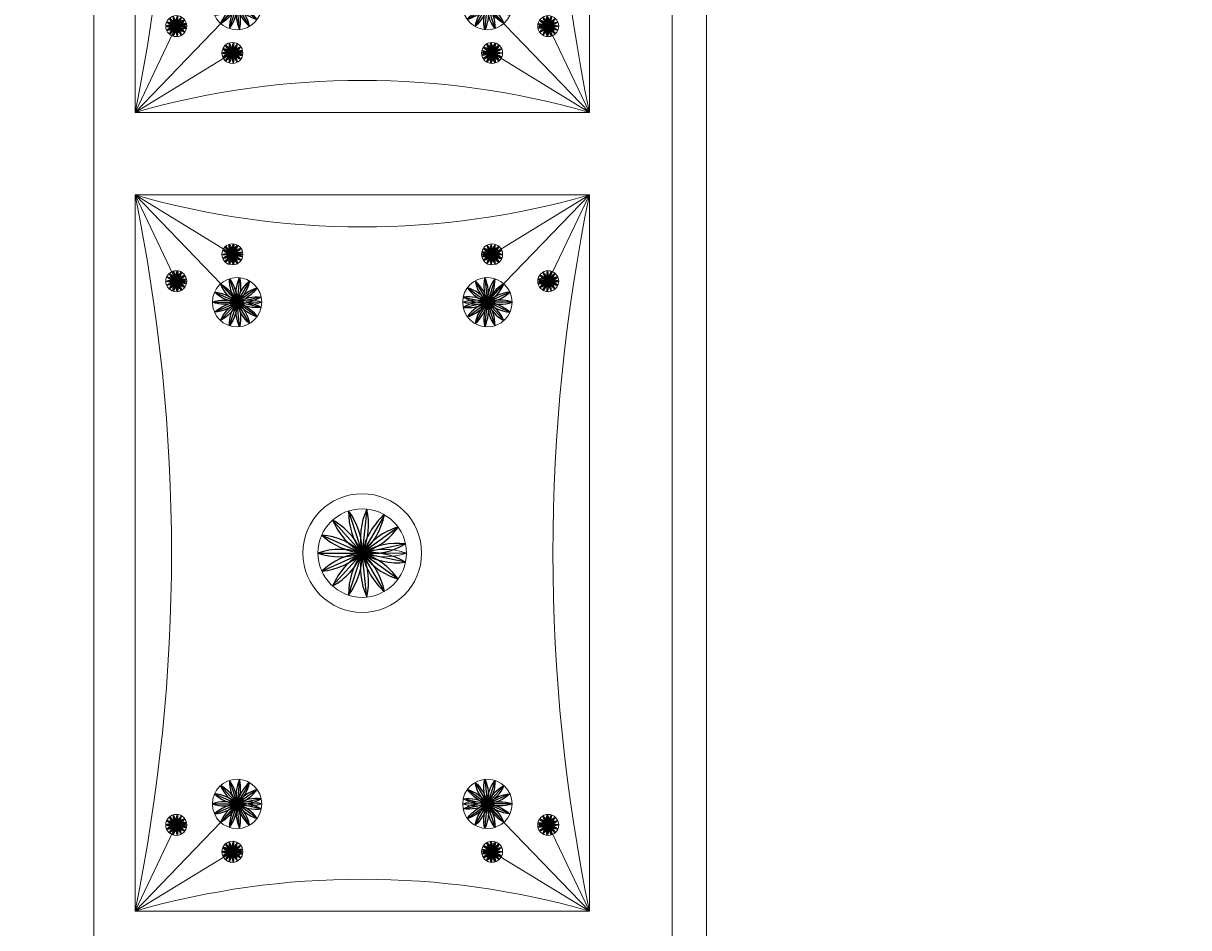
# Model space of a CAD drawing. Units: inches. Extents: x -61 to 1599, y -1316 to 257.
# Tile 147 of 204: x 406 to 440, y 74 to 101. Entities that reach past the tile are written whole.
import ezdxf

# ---------------------------------------------------------------- set-up
doc = ezdxf.new("R2010")
doc.units = ezdxf.units.IN
doc.header["$MEASUREMENT"] = 0
doc.layers.add('A-ANNO-DIMS', color=2, linetype='Continuous', lineweight=18)
doc.layers.add('FURNITURE', color=83, linetype='Continuous', lineweight=18)
doc.layers.add('LT', color=8, linetype='Continuous')
doc.styles.get("Standard").update_dxf_attribs({"font": 'arial.ttf'})
doc.dimstyles.get("Standard").update_dxf_attribs({"dimtxt": 0.18, "dimasz": 0.18, "dimexe": 0.18, "dimexo": 0.0625, "dimgap": 0.09, "dimtad": 0, "dimtih": 1, "dimtoh": 1, "dimdec": 0, "dimzin": 0, "dimdsep": 46, "dimlunit": 3, "dimtxsty": 'Standard', "dimcen": 0.09, "dimadec": 0, "dimazin": 0, "dimtfac": 1, "dimtdec": 0, "dimtofl": 0, "dimtmove": 0, "dimatfit": 3, "dimfxl": 1, "dimtolj": 1, "dimtzin": 0, "dimarcsym": 0})

# ---------------------------------------------------------------- blocks, each defined once
blk = doc.blocks.new('*U100')
at = {"layer": 'LT'}
blk.add_line((0, 0.152), (0, -0.152), dxfattribs=at)
for centre, start, end in [((0.443, 0), 160.9983, 199.0017), ((-0.443, 0), 340.9983, 19.0017)]:
    blk.add_arc(centre, 0.468, start, end, dxfattribs=at)
blk = doc.blocks.new('*U101')
at = {"layer": 'LT', "transparency": 16777216}
for p, rotation in [((-57.958, -16.311), 72), ((-57.926, -16.256), 48.00000000000001), ((-57.875, -16.219), 24), ((-57.751, -16.219), 336), ((-57.699, -16.256), 312), ((-57.668, -16.311), 288), ((-57.964, -16.374), 96), ((-57.945, -16.435), 120), ((-57.902, -16.482), 144), ((-57.844, -16.508), 168.0000000000001), ((-57.781, -16.508), 192), ((-57.723, -16.482), 216), ((-57.68, -16.435), 240), ((-57.661, -16.374), 264)]:
    blk.add_blockref('*U100', p, dxfattribs=dict(at, rotation=rotation))
blk.add_blockref('*U100', (-57.813, -16.206), dxfattribs=at)
blk = doc.blocks.new('*U104')
at = {"layer": 'LT'}
blk.add_line((0, 0.152), (0, -0.152), dxfattribs=at)
for centre, start, end in [((0.443, 0), 160.9983, 199.0017), ((-0.443, 0), 340.9983, 19.0017)]:
    blk.add_arc(centre, 0.468, start, end, dxfattribs=at)
blk = doc.blocks.new('*U105')
at = {"layer": 'LT', "transparency": 16777216}
for p, rotation in [((-57.958, -16.311), 72), ((-57.926, -16.256), 48.00000000000001), ((-57.875, -16.219), 24), ((-57.751, -16.219), 336), ((-57.699, -16.256), 312), ((-57.668, -16.311), 288), ((-57.964, -16.374), 96), ((-57.945, -16.435), 120), ((-57.902, -16.482), 144), ((-57.844, -16.508), 168.0000000000001), ((-57.781, -16.508), 192), ((-57.723, -16.482), 216), ((-57.68, -16.435), 240), ((-57.661, -16.374), 264)]:
    blk.add_blockref('*U104', p, dxfattribs=dict(at, rotation=rotation))
blk.add_blockref('*U104', (-57.813, -16.206), dxfattribs=at)
blk = doc.blocks.new('*U71')
at = {"layer": 'LT'}
blk.add_line((0, 0.152), (0, -0.152), dxfattribs=at)
for centre, start, end in [((0.443, 0), 160.9983, 199.0017), ((-0.443, 0), 340.9983, 19.0017)]:
    blk.add_arc(centre, 0.468, start, end, dxfattribs=at)
blk = doc.blocks.new('*U58')
at = {"layer": 'LT', "transparency": 16777216}
for p, rotation in [((-57.958, -16.311), 72), ((-57.926, -16.256), 48.00000000000001), ((-57.875, -16.219), 24), ((-57.751, -16.219), 336), ((-57.699, -16.256), 312), ((-57.668, -16.311), 288), ((-57.964, -16.374), 96), ((-57.945, -16.435), 120), ((-57.902, -16.482), 144), ((-57.844, -16.508), 168.0000000000001), ((-57.781, -16.508), 192), ((-57.723, -16.482), 216), ((-57.68, -16.435), 240), ((-57.661, -16.374), 264)]:
    blk.add_blockref('*U71', p, dxfattribs=dict(at, rotation=rotation))
blk.add_blockref('*U71', (-57.813, -16.206), dxfattribs=at)
blk = doc.blocks.new('*U94')
at = {"layer": 'LT'}
blk.add_line((0, 0.359), (0, -0.359), dxfattribs=at)
for centre, start, end in [((1.041, 0), 160.9983, 199.0017), ((-1.041, 0), 340.9983, 19.0017)]:
    blk.add_arc(centre, 1.101, start, end, dxfattribs=at)
blk = doc.blocks.new('*U95')
at = {"layer": 'LT', "transparency": 16777216}
for p, rotation in [((-136.107, -38.143), 23.99999999999999), ((-135.815, -38.143), 336.0000000000001), ((-136.302, -38.36), 72), ((-136.227, -38.231), 48.00000000000001), ((-135.694, -38.231), 312), ((-135.62, -38.36), 288.0000000000001), ((-136.318, -38.508), 96), ((-136.271, -38.65), 120), ((-136.172, -38.761), 144), ((-136.035, -38.822), 168.0000000000001), ((-135.886, -38.822), 191.9999999999999), ((-135.75, -38.761), 216), ((-135.65, -38.65), 240), ((-135.604, -38.508), 264)]:
    blk.add_blockref('*U94', p, dxfattribs=dict(at, rotation=rotation))
blk.add_blockref('*U94', (-135.961, -38.112), dxfattribs=at)
blk = doc.blocks.new('*U57')
at = {"layer": 'LT'}
blk.add_line((0, 0.359), (0, -0.359), dxfattribs=at)
for centre, start, end in [((1.041, 0), 160.9983, 199.0017), ((-1.041, 0), 340.9983, 19.0017)]:
    blk.add_arc(centre, 1.101, start, end, dxfattribs=at)
blk = doc.blocks.new('*U99')
at = {"layer": 'LT', "transparency": 16777216}
for p, rotation in [((-136.107, -38.143), 23.99999999999999), ((-135.815, -38.143), 336.0000000000001), ((-136.302, -38.36), 72), ((-136.227, -38.231), 48.00000000000001), ((-135.694, -38.231), 312), ((-135.62, -38.36), 288.0000000000001), ((-136.318, -38.508), 96), ((-136.271, -38.65), 120), ((-136.172, -38.761), 144), ((-136.035, -38.822), 168.0000000000001), ((-135.886, -38.822), 191.9999999999999), ((-135.75, -38.761), 216), ((-135.65, -38.65), 240), ((-135.604, -38.508), 264)]:
    blk.add_blockref('*U57', p, dxfattribs=dict(at, rotation=rotation))
blk.add_blockref('*U57', (-135.961, -38.112), dxfattribs=at)
blk = doc.blocks.new('*U80')
at = {"layer": 'LT'}
blk.add_line((0, 0.359), (0, -0.359), dxfattribs=at)
for centre, start, end in [((1.041, 0), 160.9983, 199.0017), ((-1.041, 0), 340.9983, 19.0017)]:
    blk.add_arc(centre, 1.101, start, end, dxfattribs=at)
blk = doc.blocks.new('*U96')
at = {"layer": 'LT', "transparency": 16777216}
for p, rotation in [((-136.107, -38.143), 23.99999999999999), ((-135.815, -38.143), 336.0000000000001), ((-136.302, -38.36), 72), ((-136.227, -38.231), 48.00000000000001), ((-135.694, -38.231), 312), ((-135.62, -38.36), 288.0000000000001), ((-136.318, -38.508), 96), ((-136.271, -38.65), 120), ((-136.172, -38.761), 144), ((-136.035, -38.822), 168.0000000000001), ((-135.886, -38.822), 191.9999999999999), ((-135.75, -38.761), 216), ((-135.65, -38.65), 240), ((-135.604, -38.508), 264)]:
    blk.add_blockref('*U80', p, dxfattribs=dict(at, rotation=rotation))
blk.add_blockref('*U80', (-135.961, -38.112), dxfattribs=at)
blk = doc.blocks.new('*U102')
at = {"layer": 'LT'}
blk.add_line((0, 0.152), (0, -0.152), dxfattribs=at)
for centre, start, end in [((0.443, 0), 160.9983, 199.0017), ((-0.443, 0), 340.9983, 19.0017)]:
    blk.add_arc(centre, 0.468, start, end, dxfattribs=at)
blk = doc.blocks.new('*U103')
at = {"layer": 'LT', "transparency": 16777216}
for p, rotation in [((-57.958, -16.311), 72), ((-57.926, -16.256), 48.00000000000001), ((-57.875, -16.219), 24), ((-57.751, -16.219), 336), ((-57.699, -16.256), 312), ((-57.668, -16.311), 288), ((-57.964, -16.374), 96), ((-57.945, -16.435), 120), ((-57.902, -16.482), 144), ((-57.844, -16.508), 168.0000000000001), ((-57.781, -16.508), 192), ((-57.723, -16.482), 216), ((-57.68, -16.435), 240), ((-57.661, -16.374), 264)]:
    blk.add_blockref('*U102', p, dxfattribs=dict(at, rotation=rotation))
blk.add_blockref('*U102', (-57.813, -16.206), dxfattribs=at)
blk = doc.blocks.new('*U55')
at = {"layer": 'LT'}
blk.add_line((0, 0.152), (0, -0.152), dxfattribs=at)
for centre, start, end in [((0.443, 0), 160.9983, 199.0017), ((-0.443, 0), 340.9983, 19.0017)]:
    blk.add_arc(centre, 0.468, start, end, dxfattribs=at)
blk = doc.blocks.new('*U56')
at = {"layer": 'LT', "transparency": 16777216}
for p, rotation in [((-57.958, -16.311), 72), ((-57.926, -16.256), 48.00000000000001), ((-57.875, -16.219), 24), ((-57.751, -16.219), 336), ((-57.699, -16.256), 312), ((-57.668, -16.311), 288), ((-57.964, -16.374), 96), ((-57.945, -16.435), 120), ((-57.902, -16.482), 144), ((-57.844, -16.508), 168.0000000000001), ((-57.781, -16.508), 192), ((-57.723, -16.482), 216), ((-57.68, -16.435), 240), ((-57.661, -16.374), 264)]:
    blk.add_blockref('*U55', p, dxfattribs=dict(at, rotation=rotation))
blk.add_blockref('*U55', (-57.813, -16.206), dxfattribs=at)
blk = doc.blocks.new('*U59')
at = {"layer": 'LT'}
blk.add_line((0, 0.152), (0, -0.152), dxfattribs=at)
for centre, start, end in [((0.443, 0), 160.9983, 199.0017), ((-0.443, 0), 340.9983, 19.0017)]:
    blk.add_arc(centre, 0.468, start, end, dxfattribs=at)
blk = doc.blocks.new('*U60')
at = {"layer": 'LT', "transparency": 16777216}
for p, rotation in [((-57.958, -16.311), 72), ((-57.926, -16.256), 48.00000000000001), ((-57.875, -16.219), 24), ((-57.751, -16.219), 336), ((-57.699, -16.256), 312), ((-57.668, -16.311), 288), ((-57.964, -16.374), 96), ((-57.945, -16.435), 120), ((-57.902, -16.482), 144), ((-57.844, -16.508), 168.0000000000001), ((-57.781, -16.508), 192), ((-57.723, -16.482), 216), ((-57.68, -16.435), 240), ((-57.661, -16.374), 264)]:
    blk.add_blockref('*U59', p, dxfattribs=dict(at, rotation=rotation))
blk.add_blockref('*U59', (-57.813, -16.206), dxfattribs=at)
blk = doc.blocks.new('*U106')
at = {"layer": 'LT'}
blk.add_line((0, 0.643), (0, -0.643), dxfattribs=at)
for centre, start, end in [((1.867, 0), 160.9983, 199.0017), ((-1.867, 0), 340.9983, 19.0017)]:
    blk.add_arc(centre, 1.975, start, end, dxfattribs=at)
blk = doc.blocks.new('*U93')
at = {"layer": 'LT', "transparency": 16777216}
blk.add_blockref('*U106', (-243.723, -68.32), dxfattribs=at)
for p, rotation in [((-244.201, -68.532), 48.00000000000001), ((-243.984, -68.375), 23.99999999999999), ((-243.461, -68.375), 336.0000000000001), ((-243.245, -68.532), 312), ((-244.334, -68.764), 72), ((-243.111, -68.764), 288), ((-244.362, -69.03), 96), ((-244.28, -69.284), 120), ((-244.101, -69.483), 144), ((-243.856, -69.591), 168), ((-243.589, -69.591), 192), ((-243.345, -69.483), 216), ((-243.166, -69.284), 240), ((-243.083, -69.03), 264)]:
    blk.add_blockref('*U106', p, dxfattribs=dict(at, rotation=rotation))
blk = doc.blocks.new('*U83')
at = {"layer": 'LT'}
blk.add_line((0, 0.359), (0, -0.359), dxfattribs=at)
for centre, start, end in [((1.041, 0), 160.9983, 199.0017), ((-1.041, 0), 340.9983, 19.0017)]:
    blk.add_arc(centre, 1.101, start, end, dxfattribs=at)
blk = doc.blocks.new('*U84')
at = {"layer": 'LT', "transparency": 16777216}
for p, rotation in [((-136.107, -38.143), 23.99999999999999), ((-135.815, -38.143), 336.0000000000001), ((-136.302, -38.36), 72), ((-136.227, -38.231), 48.00000000000001), ((-135.694, -38.231), 312), ((-135.62, -38.36), 288.0000000000001), ((-136.318, -38.508), 96), ((-136.271, -38.65), 120), ((-136.172, -38.761), 144), ((-136.035, -38.822), 168.0000000000001), ((-135.886, -38.822), 191.9999999999999), ((-135.75, -38.761), 216), ((-135.65, -38.65), 240), ((-135.604, -38.508), 264)]:
    blk.add_blockref('*U83', p, dxfattribs=dict(at, rotation=rotation))
blk.add_blockref('*U83', (-135.961, -38.112), dxfattribs=at)
blk = doc.blocks.new('*U74')
at = {"layer": 'LT'}
blk.add_line((0, 0.359), (0, -0.359), dxfattribs=at)
for centre, start, end in [((1.041, 0), 160.9983, 199.0017), ((-1.041, 0), 340.9983, 19.0017)]:
    blk.add_arc(centre, 1.101, start, end, dxfattribs=at)
blk = doc.blocks.new('*U75')
at = {"layer": 'LT', "transparency": 16777216}
for p, rotation in [((-136.107, -38.143), 23.99999999999999), ((-135.815, -38.143), 336.0000000000001), ((-136.302, -38.36), 72), ((-136.227, -38.231), 48.00000000000001), ((-135.694, -38.231), 312), ((-135.62, -38.36), 288.0000000000001), ((-136.318, -38.508), 96), ((-136.271, -38.65), 120), ((-136.172, -38.761), 144), ((-136.035, -38.822), 168.0000000000001), ((-135.886, -38.822), 191.9999999999999), ((-135.75, -38.761), 216), ((-135.65, -38.65), 240), ((-135.604, -38.508), 264)]:
    blk.add_blockref('*U74', p, dxfattribs=dict(at, rotation=rotation))
blk.add_blockref('*U74', (-135.961, -38.112), dxfattribs=at)
blk = doc.blocks.new('*U65')
at = {"layer": 'LT'}
blk.add_line((0, 0.359), (0, -0.359), dxfattribs=at)
for centre, start, end in [((1.041, 0), 160.9983, 199.0017), ((-1.041, 0), 340.9983, 19.0017)]:
    blk.add_arc(centre, 1.101, start, end, dxfattribs=at)
blk = doc.blocks.new('*U66')
at = {"layer": 'LT', "transparency": 16777216}
for p, rotation in [((-136.107, -38.143), 23.99999999999999), ((-135.815, -38.143), 336.0000000000001), ((-136.302, -38.36), 72), ((-136.227, -38.231), 48.00000000000001), ((-135.694, -38.231), 312), ((-135.62, -38.36), 288.0000000000001), ((-136.318, -38.508), 96), ((-136.271, -38.65), 120), ((-136.172, -38.761), 144), ((-136.035, -38.822), 168.0000000000001), ((-135.886, -38.822), 191.9999999999999), ((-135.75, -38.761), 216), ((-135.65, -38.65), 240), ((-135.604, -38.508), 264)]:
    blk.add_blockref('*U65', p, dxfattribs=dict(at, rotation=rotation))
blk.add_blockref('*U65', (-135.961, -38.112), dxfattribs=at)
blk = doc.blocks.new('*U78')
at = {"layer": 'LT'}
blk.add_line((0, 0.152), (0, -0.152), dxfattribs=at)
for centre, start, end in [((0.443, 0), 160.9983, 199.0017), ((-0.443, 0), 340.9983, 19.0017)]:
    blk.add_arc(centre, 0.468, start, end, dxfattribs=at)
blk = doc.blocks.new('*U79')
at = {"layer": 'LT', "transparency": 16777216}
for p, rotation in [((-57.958, -16.311), 72), ((-57.926, -16.256), 48.00000000000001), ((-57.875, -16.219), 24), ((-57.751, -16.219), 336), ((-57.699, -16.256), 312), ((-57.668, -16.311), 288), ((-57.964, -16.374), 96), ((-57.945, -16.435), 120), ((-57.902, -16.482), 144), ((-57.844, -16.508), 168.0000000000001), ((-57.781, -16.508), 192), ((-57.723, -16.482), 216), ((-57.68, -16.435), 240), ((-57.661, -16.374), 264)]:
    blk.add_blockref('*U78', p, dxfattribs=dict(at, rotation=rotation))
blk.add_blockref('*U78', (-57.813, -16.206), dxfattribs=at)
blk = doc.blocks.new('*U72')
at = {"layer": 'LT'}
blk.add_line((0, 0.152), (0, -0.152), dxfattribs=at)
for centre, start, end in [((0.443, 0), 160.9983, 199.0017), ((-0.443, 0), 340.9983, 19.0017)]:
    blk.add_arc(centre, 0.468, start, end, dxfattribs=at)
blk = doc.blocks.new('*U73')
at = {"layer": 'LT', "transparency": 16777216}
for p, rotation in [((-57.958, -16.311), 72), ((-57.926, -16.256), 48.00000000000001), ((-57.875, -16.219), 24), ((-57.751, -16.219), 336), ((-57.699, -16.256), 312), ((-57.668, -16.311), 288), ((-57.964, -16.374), 96), ((-57.945, -16.435), 120), ((-57.902, -16.482), 144), ((-57.844, -16.508), 168.0000000000001), ((-57.781, -16.508), 192), ((-57.723, -16.482), 216), ((-57.68, -16.435), 240), ((-57.661, -16.374), 264)]:
    blk.add_blockref('*U72', p, dxfattribs=dict(at, rotation=rotation))
blk.add_blockref('*U72', (-57.813, -16.206), dxfattribs=at)
blk = doc.blocks.new('*U89')
at = {"layer": 'LT'}
blk.add_line((0, 0.152), (0, -0.152), dxfattribs=at)
for centre, start, end in [((0.443, 0), 160.9983, 199.0017), ((-0.443, 0), 340.9983, 19.0017)]:
    blk.add_arc(centre, 0.468, start, end, dxfattribs=at)
blk = doc.blocks.new('*U90')
at = {"layer": 'LT', "transparency": 16777216}
for p, rotation in [((-57.958, -16.311), 72), ((-57.926, -16.256), 48.00000000000001), ((-57.875, -16.219), 24), ((-57.751, -16.219), 336), ((-57.699, -16.256), 312), ((-57.668, -16.311), 288), ((-57.964, -16.374), 96), ((-57.945, -16.435), 120), ((-57.902, -16.482), 144), ((-57.844, -16.508), 168.0000000000001), ((-57.781, -16.508), 192), ((-57.723, -16.482), 216), ((-57.68, -16.435), 240), ((-57.661, -16.374), 264)]:
    blk.add_blockref('*U89', p, dxfattribs=dict(at, rotation=rotation))
blk.add_blockref('*U89', (-57.813, -16.206), dxfattribs=at)
blk = doc.blocks.new('*U76')
at = {"layer": 'LT'}
blk.add_line((0, 0.152), (0, -0.152), dxfattribs=at)
for centre, start, end in [((0.443, 0), 160.9983, 199.0017), ((-0.443, 0), 340.9983, 19.0017)]:
    blk.add_arc(centre, 0.468, start, end, dxfattribs=at)
blk = doc.blocks.new('*U77')
at = {"layer": 'LT', "transparency": 16777216}
for p, rotation in [((-57.958, -16.311), 72), ((-57.926, -16.256), 48.00000000000001), ((-57.875, -16.219), 24), ((-57.751, -16.219), 336), ((-57.699, -16.256), 312), ((-57.668, -16.311), 288), ((-57.964, -16.374), 96), ((-57.945, -16.435), 120), ((-57.902, -16.482), 144), ((-57.844, -16.508), 168.0000000000001), ((-57.781, -16.508), 192), ((-57.723, -16.482), 216), ((-57.68, -16.435), 240), ((-57.661, -16.374), 264)]:
    blk.add_blockref('*U76', p, dxfattribs=dict(at, rotation=rotation))
blk.add_blockref('*U76', (-57.813, -16.206), dxfattribs=at)
blk = doc.blocks.new('*U81')
at = {"layer": 'LT'}
blk.add_line((0, 0.152), (0, -0.152), dxfattribs=at)
for centre, start, end in [((0.443, 0), 160.9983, 199.0017), ((-0.443, 0), 340.9983, 19.0017)]:
    blk.add_arc(centre, 0.468, start, end, dxfattribs=at)
blk = doc.blocks.new('*U82')
at = {"layer": 'LT', "transparency": 16777216}
for p, rotation in [((-57.958, -16.311), 72), ((-57.926, -16.256), 48.00000000000001), ((-57.875, -16.219), 24), ((-57.751, -16.219), 336), ((-57.699, -16.256), 312), ((-57.668, -16.311), 288), ((-57.964, -16.374), 96), ((-57.945, -16.435), 120), ((-57.902, -16.482), 144), ((-57.844, -16.508), 168.0000000000001), ((-57.781, -16.508), 192), ((-57.723, -16.482), 216), ((-57.68, -16.435), 240), ((-57.661, -16.374), 264)]:
    blk.add_blockref('*U81', p, dxfattribs=dict(at, rotation=rotation))
blk.add_blockref('*U81', (-57.813, -16.206), dxfattribs=at)
blk = doc.blocks.new('*U87')
at = {"layer": 'LT'}
blk.add_line((0, 0.152), (0, -0.152), dxfattribs=at)
for centre, start, end in [((0.443, 0), 160.9983, 199.0017), ((-0.443, 0), 340.9983, 19.0017)]:
    blk.add_arc(centre, 0.468, start, end, dxfattribs=at)
blk = doc.blocks.new('*U88')
at = {"layer": 'LT', "transparency": 16777216}
for p, rotation in [((-57.958, -16.311), 72), ((-57.926, -16.256), 48.00000000000001), ((-57.875, -16.219), 24), ((-57.751, -16.219), 336), ((-57.699, -16.256), 312), ((-57.668, -16.311), 288), ((-57.964, -16.374), 96), ((-57.945, -16.435), 120), ((-57.902, -16.482), 144), ((-57.844, -16.508), 168.0000000000001), ((-57.781, -16.508), 192), ((-57.723, -16.482), 216), ((-57.68, -16.435), 240), ((-57.661, -16.374), 264)]:
    blk.add_blockref('*U87', p, dxfattribs=dict(at, rotation=rotation))
blk.add_blockref('*U87', (-57.813, -16.206), dxfattribs=at)
blk = doc.blocks.new('BED-DOUBLE-COMPACT')
for p, q in [((16.8, 60.036), (16.8, 0.036)), ((17.8, 60.036), (17.8, 0.036)), ((14.4, 31.236), (14.4, 52.036)), ((1.2, 31.236), (4.201, 34.339)), ((14.4, 31.236), (11.4, 34.339)), ((1.2, 31.236), (2.398, 33.74)), ((2.398, 33.74), (2.703, 33.74)), ((13.203, 33.74), (12.898, 33.74)), ((14.4, 31.236), (13.203, 33.74)), ((1.2, 31.236), (4.028, 32.961)), ((4.028, 32.961), (4.333, 32.961)), ((11.572, 32.961), (11.267, 32.961)), ((14.4, 31.236), (11.572, 32.961)), ((1.2, 31.236), (1.2, 31.236)), ((1.2, 28.836), (14.4, 28.836)), ((1.2, 28.836), (2.398, 26.332)), ((1.2, 28.836), (4.201, 25.734)), ((1.2, 28.836), (4.028, 27.112)), ((14.4, 28.836), (11.4, 25.734)), ((14.4, 28.836), (11.572, 27.112)), ((14.4, 28.836), (13.203, 26.332)), ((14.4, 8.036), (14.4, 28.836)), ((4.028, 27.112), (4.333, 27.112)), ((11.572, 27.112), (11.267, 27.112)), ((2.398, 26.332), (2.703, 26.332)), ((13.203, 26.332), (12.898, 26.332)), ((4.165, 25.722), (4.882, 25.722)), ((11.436, 25.722), (10.719, 25.722)), ((7.8, 18.436), (9.086, 18.436)), ((1.2, 8.036), (4.201, 11.139)), ((4.165, 11.151), (4.882, 11.151)), ((11.436, 11.151), (10.719, 11.151)), ((14.4, 8.036), (11.4, 11.139)), ((1.2, 8.036), (2.398, 10.54)), ((2.398, 10.54), (2.703, 10.54)), ((13.203, 10.54), (12.898, 10.54)), ((14.4, 8.036), (13.203, 10.54)), ((1.2, 8.036), (4.028, 9.761)), ((4.028, 9.761), (4.333, 9.761)), ((11.572, 9.761), (11.267, 9.761)), ((14.4, 8.036), (11.572, 9.761)), ((1.2, 8.036), (1.2, 8.036))]:
    blk.add_line(p, q)
for points in [[(77, 60.036), (3, 60.036, 0.414214), (0, 57.036), (0, 3.036, 0.414214), (3, 0.036), (77, 0.036, 0.414214), (80, 3.036), (80, 57.036, 0.414214)], [(2.398, 33.74, 0.167358), (2.703, 33.74, 0.167358)], [(4.028, 32.961, 0.167358), (4.333, 32.961, 0.167358)], [(11.267, 32.961, 0.167358), (11.572, 32.961, 0.167358)], [(4.333, 27.112, 0.167358), (4.028, 27.112, 0.167358)], [(11.572, 27.112, 0.167358), (11.267, 27.112, 0.167358)], [(2.703, 26.332, 0.167358), (2.398, 26.332, 0.167358)], [(13.203, 26.332, 0.167358), (12.898, 26.332, 0.167358)], [(4.882, 25.722, 0.167358), (4.165, 25.722, 0.167358)], [(11.436, 25.722, 0.167358), (10.719, 25.722, 0.167358)], [(7.8, 18.436, 0.167358), (9.086, 18.436, 0.167358)], [(4.165, 11.151, 0.167358), (4.882, 11.151, 0.167358)], [(10.719, 11.151, 0.167358), (11.436, 11.151, 0.167358)], [(2.398, 10.54, 0.167358), (2.703, 10.54, 0.167358)], [(4.028, 9.761, 0.167358), (4.333, 9.761, 0.167358)], [(11.267, 9.761, 0.167358), (11.572, 9.761, 0.167358)]]:
    blk.add_lwpolyline(points, format="xyb", close=True)
for points in [[(14.4, 31.236), (1.2, 31.236), (1.2, 52.036), (14.4, 52.036), (14.4, 31.236), (1.2, 31.236), (1.2, 52.036)], [(14.4, 8.036), (1.2, 8.036), (1.2, 28.836)]]:
    blk.add_lwpolyline(points)
for centre, radius in [((4.165, 34.351), 0.717), ((11.436, 34.351), 0.717), ((2.398, 33.74), 0.305), ((13.203, 33.74), 0.305), ((4.028, 32.961), 0.305), ((11.572, 32.961), 0.305), ((4.028, 27.112), 0.305), ((11.572, 27.112), 0.305), ((2.398, 26.332), 0.305), ((4.165, 25.722), 0.717), ((11.436, 25.722), 0.717), ((13.203, 26.332), 0.305), ((7.8, 18.436), 1.724), ((7.8, 18.436), 1.286), ((4.165, 11.151), 0.717), ((11.436, 11.151), 0.717), ((2.398, 10.54), 0.305), ((13.203, 10.54), 0.305), ((4.028, 9.761), 0.305), ((11.572, 9.761), 0.305)]:
    blk.add_circle(centre, radius)
for centre, radius, start, end in [((-49.227, 41.636), 51.488, 348.3468, 11.6532), ((64.827, 41.636), 51.488, 168.3468, 191.6532), ((13.05, 33.298), 0.468, 70.9983, 109.0017), ((13.05, 34.183), 0.468, 250.9983, 289.0017), ((7.8, 8.212), 23.951, 74.0046, 105.9954), ((-49.227, 18.436), 51.488, 348.3468, 11.6532), ((7.8, 51.86), 23.951, 254.0046, 285.9954), ((64.827, 18.436), 51.488, 168.3468, 191.6532), ((13.05, 10.098), 0.468, 70.9983, 109.0017), ((13.05, 10.983), 0.468, 250.9983, 289.0017), ((7.8, -14.988), 23.951, 74.0046, 105.9954)]:
    blk.add_arc(centre, radius, start, end)
for name, p, rotation in [('*U96', (-34.306, 170.312), 89.99999999999999), ('*U58', (-13.96, 91.553), 89.99999999999999), ('*U60', (-12.33, 90.773), 89.99999999999999), ('*U73', (27.931, -30.701), 270), ('*U75', (49.907, -110.239), 270), ('*U82', (29.561, -31.48), 270), ('*U93', (-61.162, 262.159), 89.99999999999999), ('*U95', (-34.306, 147.112), 89.99999999999999), ('*U101', (-13.96, 68.353), 89.99999999999999), ('*U103', (-12.33, 67.573), 89.99999999999999)]:
    blk.add_blockref(name, p, dxfattribs=dict(rotation=rotation))
at = {"xscale": -1}
for name, p, rotation in [('*U66', (49.907, 170.312), 270), ('*U88', (29.561, 91.553), 270), ('*U90', (27.931, 90.773), 270), ('*U56', (-12.33, -30.701), 90), ('*U105', (-13.96, -31.48), 90), ('*U99', (-34.306, -110.239), 90), ('*U84', (49.907, 147.112), 270), ('*U77', (29.561, 68.353), 270), ('*U79', (27.931, 67.573), 270)]:
    blk.add_blockref(name, p, dxfattribs=dict(at, rotation=rotation))
blk = doc.blocks.new('*D703')
at = {"layer": 'A-ANNO-DIMS', "color": 0, "lineweight": -2, "transparency": 16777216}
for p, q in [((372.32, -616.882), (372.32, 257.457)), ((455.833, -616.882), (455.833, 257.457)), ((372.5, 257.277), (413.7, 257.277)), ((455.653, 257.277), (414.453, 257.277))]:
    blk.add_line(p, q, dxfattribs=at)
at = {"layer": 'A-ANNO-DIMS', "color": 0, "transparency": 16777216}
for points in [[(372.5, 257.307), (372.5, 257.247), (372.32, 257.277)], [(455.653, 257.307), (455.653, 257.247), (455.833, 257.277)]]:
    blk.add_solid(points, dxfattribs=at)
at = {"layer": 'DEFPOINTS', "color": 0, "transparency": 16777216}
for p in [(455.833, 257.277), (372.32, -616.945), (455.833, -616.945)]:
    blk.add_point(p, dxfattribs=at)
at = {"layer": 'A-ANNO-DIMS', "color": 0, "transparency": 16777216, "insert": (414.076, 257.277), "char_height": 0.18, "attachment_point": 5}
blk.add_mtext('\\A1;83.51', dxfattribs=at)

msp = doc.modelspace()

# ---------------------------------------------------------------- block references
at = {"layer": 'FURNITURE'}
msp.add_blockref('BED-DOUBLE-COMPACT', (407.794, 66.733), dxfattribs=at)

# ---------------------------------------------------------------- dimensions: what is measured, and where the dimension line sits
at = {"layer": 'A-ANNO-DIMS'}
dim = msp.add_linear_dim(base=(455.8327, 257.2771), p1=(372.3201, -616.9446), p2=(455.8327, -616.9446), dimstyle='Standard', override={"dimdec": 2, "dimlfac": 1, "dimrnd": 0, "dimzin": 0, "dimdsep": 46, "dimlunit": 2}, dxfattribs=at)
dim.commit()
dim.dimension.update_dxf_attribs({"geometry": '*D703', "text_midpoint": (414.0764, 257.2771)})

doc.saveas('drawing.dxf')
